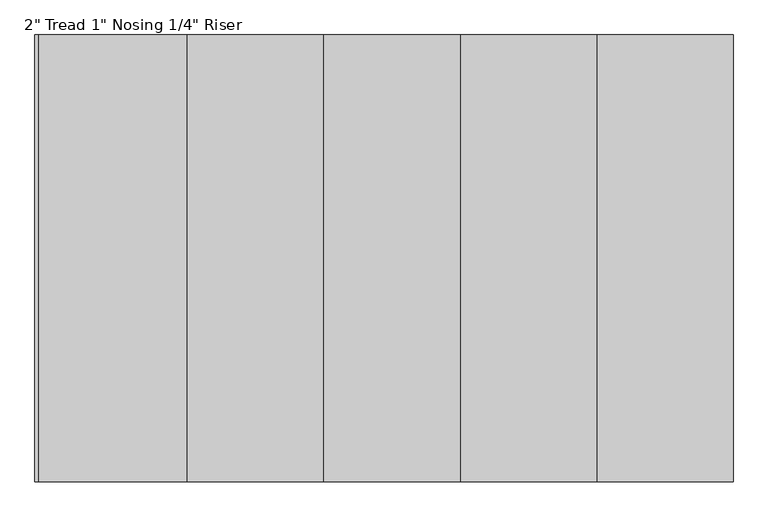
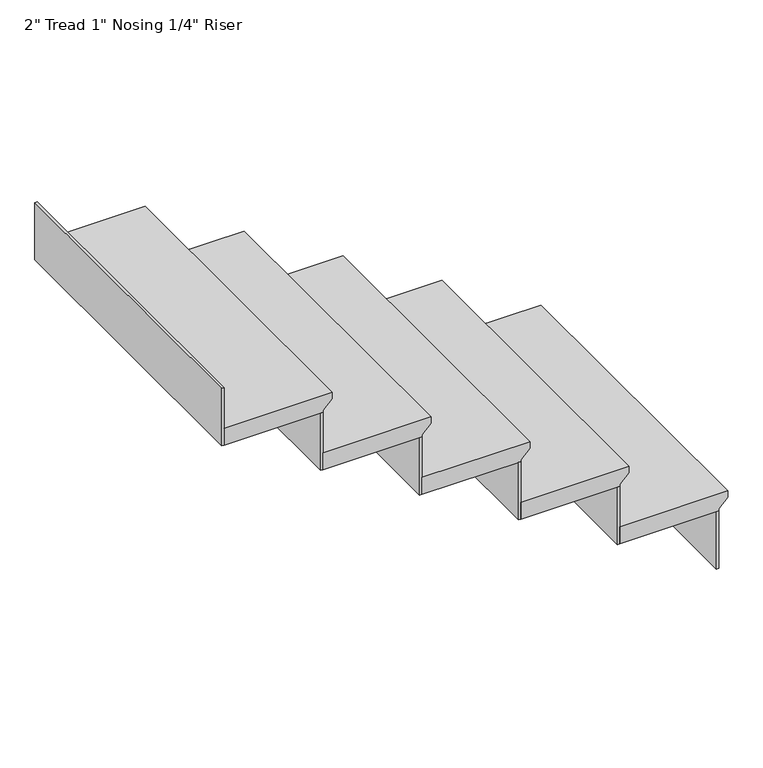
"""IFC4 building model written with IfcOpenShell, lengths in millimetres: stair flight geometry."""

from ifc_helpers import new_model, si_unit, frame, origin, place, context, project, spatial, polyline, outline, extrude, source, transform, mapped, element, save


def stair_flight_ba00a610(model_context):
    return source(origin(), model_context, "Body", "SweptSolid", [
        extrude(outline(polyline([(2190.75, -5647.5260609), (2190.75, -5952.3260609), (2139.95, -5952.3260609), (2139.95, -5672.9260609), (2146.3, -5672.9260609), (2171.7, -5647.5260609), (2190.75, -5647.5260609)])), frame((0.0, -7242.3310793, 0.0), z_axis=(0.0, 1.0, 0.0), x_axis=(0.0, 0.0, 1.0)), (0.0, 0.0, 1.0), 914.4),
        extrude(outline(polyline([(-5679.2760609, -6327.9310793), (-5672.9260609, -6327.9310793), (-5672.9260609, -7242.3310793), (-5679.2760609, -7242.3310793), (-5679.2760609, -6327.9310793)])), frame((0.0, 0.0, 1968.5), z_axis=(0.0, 0.0, 1.0), x_axis=(1.0, 0.0, 0.0)), (0.0, 0.0, 1.0), 171.45),
        extrude(outline(polyline([(-5958.6760609, -6327.9310793), (-5952.3260609, -6327.9310793), (-5952.3260609, -7242.3310793), (-5958.6760609, -7242.3310793), (-5958.6760609, -6327.9310793)])), frame((0.0, 0.0, 2139.95), z_axis=(0.0, 0.0, 1.0), x_axis=(1.0, 0.0, 0.0)), (0.0, 0.0, 1.0), 171.45),
        extrude(outline(polyline([(2362.2, -5926.9260609), (2362.2, -6231.7260609), (2311.4, -6231.7260609), (2311.4, -5952.3260609), (2317.75, -5952.3260609), (2343.15, -5926.9260609), (2362.2, -5926.9260609)])), frame((0.0, -7242.3310793, 0.0), z_axis=(0.0, 1.0, 0.0), x_axis=(0.0, 0.0, 1.0)), (0.0, 0.0, 1.0), 914.4),
        extrude(outline(polyline([(-6238.0760609, -6327.9310793), (-6231.7260609, -6327.9310793), (-6231.7260609, -7242.3310793), (-6238.0760609, -7242.3310793), (-6238.0760609, -6327.9310793)])), frame((0.0, 0.0, 2311.4), z_axis=(0.0, 0.0, 1.0), x_axis=(1.0, 0.0, 0.0)), (0.0, 0.0, 1.0), 171.45),
        extrude(outline(polyline([(2533.65, -6206.3260609), (2533.65, -6511.1260609), (2482.85, -6511.1260609), (2482.85, -6231.7260609), (2489.2, -6231.7260609), (2514.6, -6206.3260609), (2533.65, -6206.3260609)])), frame((0.0, -7242.3310793, 0.0), z_axis=(0.0, 1.0, 0.0), x_axis=(0.0, 0.0, 1.0)), (0.0, 0.0, 1.0), 914.4),
        extrude(outline(polyline([(-6517.4760609, -6327.9310793), (-6511.1260609, -6327.9310793), (-6511.1260609, -7242.3310793), (-6517.4760609, -7242.3310793), (-6517.4760609, -6327.9310793)])), frame((0.0, 0.0, 2482.85), z_axis=(0.0, 0.0, 1.0), x_axis=(1.0, 0.0, 0.0)), (0.0, 0.0, 1.0), 171.45),
        extrude(outline(polyline([(2705.1, -6485.7260609), (2705.1, -6790.5260609), (2654.3, -6790.5260609), (2654.3, -6511.1260609), (2660.65, -6511.1260609), (2686.05, -6485.7260609), (2705.1, -6485.7260609)])), frame((0.0, -7242.3310793, 0.0), z_axis=(0.0, 1.0, 0.0), x_axis=(0.0, 0.0, 1.0)), (0.0, 0.0, 1.0), 914.4),
        extrude(outline(polyline([(-6796.8760609, -6327.9310793), (-6790.5260609, -6327.9310793), (-6790.5260609, -7242.3310793), (-6796.8760609, -7242.3310793), (-6796.8760609, -6327.9310793)])), frame((0.0, 0.0, 2654.3), z_axis=(0.0, 0.0, 1.0), x_axis=(1.0, 0.0, 0.0)), (0.0, 0.0, 1.0), 171.45),
        extrude(outline(polyline([(-7076.2760609, -6327.9310793), (-7069.9260609, -6327.9310793), (-7069.9260609, -7242.3310793), (-7076.2760609, -7242.3310793), (-7076.2760609, -6327.9310793)])), frame((0.0, 0.0, 2825.75), z_axis=(0.0, 0.0, 1.0), x_axis=(1.0, 0.0, 0.0)), (0.0, 0.0, 1.0), 171.45),
        extrude(outline(polyline([(2876.55, -6765.1260609), (2876.55, -7069.9260609), (2825.75, -7069.9260609), (2825.75, -6790.5260609), (2832.1, -6790.5260609), (2857.5, -6765.1260609), (2876.55, -6765.1260609)])), frame((0.0, -7242.3310793, 0.0), z_axis=(0.0, 1.0, 0.0), x_axis=(0.0, 0.0, 1.0)), (0.0, 0.0, 1.0), 914.4),
    ])


if __name__ == "__main__":
    model = new_model("IFC4")
    model_context = context("Model", 3, world=origin())
    ifc_project = project(units=[si_unit("LENGTHUNIT", "METRE", prefix="MILLI")], contexts=[model_context])
    site = spatial("IfcSite", under=ifc_project)
    building = spatial("IfcBuilding", under=site)
    placement = place(None, origin())
    stair_flight_shape = stair_flight_ba00a610(model_context)
    element("IfcStairFlight", 1, ObjectType="2\" Tread 1\" Nosing 1/4\" Riser", at=placement, inside=building, context=model_context, shape_type="MappedRepresentation", body=[
        mapped(stair_flight_shape, transform((0.0, 0.0, 0.0), x_axis=(1.0, 0.0, 0.0), y_axis=(0.0, 1.0, 0.0), z_axis=(0.0, 0.0, 1.0))),
    ])
    save(model, "model.ifc")
